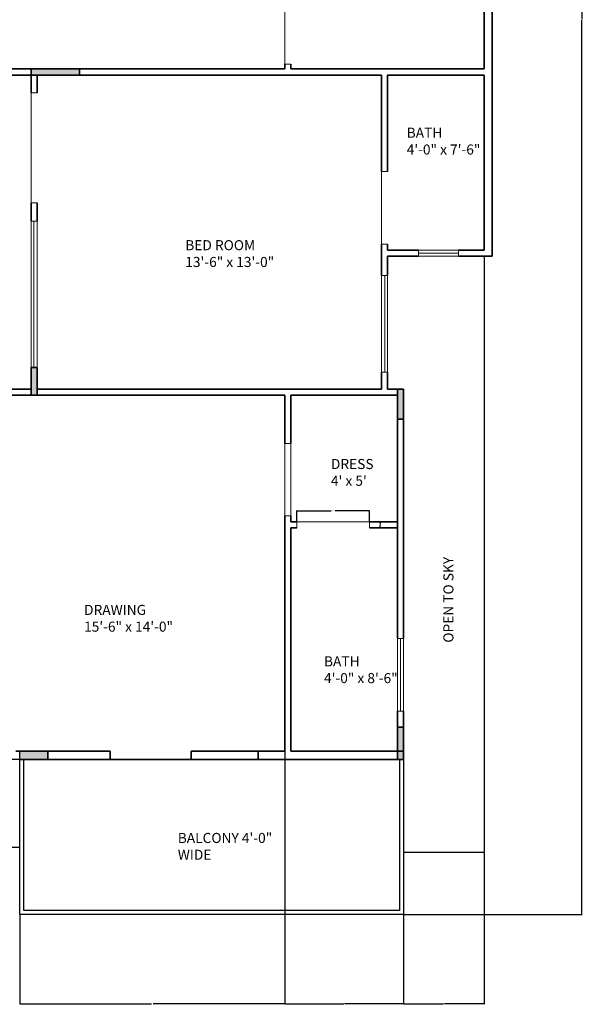
# Model space of a CAD drawing. Units: inches. Extents: x 1002 to 1561, y 1016 to 1994.
# Tile 7 of 8: x 1282 to 1561, y 1016 to 1505. Entities that reach past the tile are written whole.
import ezdxf

# ---------------------------------------------------------------- set-up
doc = ezdxf.new("R2010")
doc.units = ezdxf.units.IN
doc.header["$MEASUREMENT"] = 0
for name, color, linetype, lineweight in [('A-ANNO-DIMS', 2, 'Continuous', 18), ('A-AREA-IDEN', 7, 'Continuous', 18), ('A-WALL', 7, 'Continuous', 35), ('A-WALL-PATT', 7, 'Continuous', 13)]:
    doc.layers.add(name, color=color, linetype=linetype, lineweight=lineweight)
for name, color, linetype, lineweight, true_color in [('A-DOOR', 30, 'Continuous', 18, 0xf8991e), ('A-FLOR-EDGE', 217, 'Continuous', 25, 0x93278f), ('A-GLAZ', 217, 'Continuous', 18, 0x93278f)]:
    doc.layers.add(name, color=color, linetype=linetype, lineweight=lineweight, true_color=true_color)
doc.styles.get("Standard").update_dxf_attribs({"font": 'arial.ttf'})
doc.dimstyles.get("Standard").update_dxf_attribs({"dimtxt": 0.18, "dimasz": 0.18, "dimexe": 0.18, "dimexo": 0.0625, "dimgap": 0.09, "dimtad": 0, "dimtih": 1, "dimtoh": 1, "dimdec": 4, "dimzin": 0, "dimdsep": 46, "dimtxsty": 'Standard', "dimcen": 0.09, "dimadec": 0, "dimazin": 0, "dimtfac": 1, "dimtdec": 4, "dimtofl": 0, "dimtmove": 0, "dimatfit": 3, "dimfxl": 1, "dimtolj": 1, "dimtzin": 0, "dimarcsym": 0})

# ---------------------------------------------------------------- blocks, each defined once
blk = doc.blocks.new('DOOR-OPENING-36IN')
for p, q in [((0, 36), (3, 36)), ((0, 36), (0, 0)), ((0, 0), (3, 0))]:
    blk.add_line(p, q)
blk = doc.blocks.new('*D3')
at = {"layer": 'A-ANNO-DIMS', "color": 0, "lineweight": -2, "transparency": 16777216}
for p, q in [((1419.43, 1255.57), (1419.43, 1261.09)), ((1419.61, 1260.91), (1436.5, 1260.91)), ((1455.25, 1260.91), (1438.37, 1260.91)), ((1455.43, 1255.57), (1455.43, 1261.09))]:
    blk.add_line(p, q, dxfattribs=at)
at = {"layer": 'A-ANNO-DIMS', "color": 0, "transparency": 16777216}
for points in [[(1419.61, 1260.94), (1419.61, 1260.88), (1419.43, 1260.91)], [(1455.25, 1260.94), (1455.25, 1260.88), (1455.43, 1260.91)]]:
    blk.add_solid(points, dxfattribs=at)
at = {"layer": 'Defpoints', "color": 0, "transparency": 16777216}
for p in [(1455.43, 1260.91), (1419.43, 1255.51), (1455.43, 1255.51)]:
    blk.add_point(p, dxfattribs=at)
at = {"layer": 'A-ANNO-DIMS', "color": 0, "transparency": 16777216, "insert": (1437.43, 1260.91), "char_height": 0.18, "attachment_point": 5}
blk.add_mtext('\\A1;DOOR 36 TYP.', dxfattribs=at)
blk = doc.blocks.new('*D4')
at = {"layer": 'A-ANNO-DIMS', "color": 0, "lineweight": -2, "transparency": 16777216}
for p, q in [((1455.5, 1255.51), (1461.01, 1255.51)), ((1455.5, 1252.51), (1461.01, 1252.51)), ((1460.83, 1255.33), (1460.83, 1254.19)), ((1460.83, 1252.69), (1460.83, 1253.83))]:
    blk.add_line(p, q, dxfattribs=at)
at = {"layer": 'A-ANNO-DIMS', "color": 0, "transparency": 16777216}
for points in [[(1460.8, 1255.33), (1460.86, 1255.33), (1460.83, 1255.51)], [(1460.8, 1252.69), (1460.86, 1252.69), (1460.83, 1252.51)]]:
    blk.add_solid(points, dxfattribs=at)
at = {"layer": 'Defpoints', "color": 0, "transparency": 16777216}
for p in [(1455.43, 1255.51), (1455.43, 1252.51), (1460.83, 1252.51)]:
    blk.add_point(p, dxfattribs=at)
at = {"layer": 'A-ANNO-DIMS', "color": 0, "transparency": 16777216, "insert": (1460.83, 1254.01), "char_height": 0.18, "attachment_point": 5}
blk.add_mtext('\\A1;3 TYP.', dxfattribs=at)
blk = doc.blocks.new('*D8')
at = {"layer": 'A-ANNO-DIMS', "color": 0, "lineweight": -2, "transparency": 16777216}
for p, q in [((1516.5, 1949.51), (1561.12, 1949.51)), ((1560.94, 1949.33), (1560.94, 1505.18)), ((1560.94, 1060.67), (1560.94, 1504.82)), ((1472.5, 1060.49), (1561.12, 1060.49))]:
    blk.add_line(p, q, dxfattribs=at)
at = {"layer": 'A-ANNO-DIMS', "color": 0, "transparency": 16777216}
for points in [[(1560.91, 1949.33), (1560.97, 1949.33), (1560.94, 1949.51)], [(1560.91, 1060.67), (1560.97, 1060.67), (1560.94, 1060.49)]]:
    blk.add_solid(points, dxfattribs=at)
at = {"layer": 'Defpoints', "color": 0, "transparency": 16777216}
for p in [(1516.43, 1949.51), (1560.94, 1949.51), (1472.43, 1060.49)]:
    blk.add_point(p, dxfattribs=at)
at = {"layer": 'A-ANNO-DIMS', "color": 0, "transparency": 16777216, "insert": (1560.94, 1505), "char_height": 0.18, "attachment_point": 5}
blk.add_mtext('\\A1;889', dxfattribs=at)
blk = doc.blocks.new('*D19')
at = {"layer": 'A-ANNO-DIMS', "color": 0, "lineweight": -2, "transparency": 16777216}
for p, q in [((1413.43, 1141.45), (1413.43, 1015.8)), ((1281.79, 1060.43), (1281.79, 1015.8)), ((1281.97, 1015.98), (1347.16, 1015.98)), ((1413.25, 1015.98), (1348.07, 1015.98))]:
    blk.add_line(p, q, dxfattribs=at)
at = {"layer": 'A-ANNO-DIMS', "color": 0, "transparency": 16777216}
for points in [[(1281.97, 1016.01), (1281.97, 1015.95), (1281.79, 1015.98)], [(1413.25, 1016.01), (1413.25, 1015.95), (1413.43, 1015.98)]]:
    blk.add_solid(points, dxfattribs=at)
at = {"layer": 'Defpoints', "color": 0, "transparency": 16777216}
for p in [(1413.43, 1141.51), (1281.79, 1060.49), (1413.43, 1015.98)]:
    blk.add_point(p, dxfattribs=at)
at = {"layer": 'A-ANNO-DIMS', "color": 0, "transparency": 16777216, "insert": (1347.61, 1015.98), "char_height": 0.18, "attachment_point": 5}
blk.add_mtext('\\A1;131.64', dxfattribs=at)
blk = doc.blocks.new('*D20')
at = {"layer": 'A-ANNO-DIMS', "color": 0, "lineweight": -2, "transparency": 16777216}
for p, q in [((1413.43, 1141.45), (1413.43, 1015.8)), ((1472.43, 1060.43), (1472.43, 1015.8)), ((1413.61, 1015.98), (1442.71, 1015.98)), ((1472.25, 1015.98), (1443.15, 1015.98))]:
    blk.add_line(p, q, dxfattribs=at)
at = {"layer": 'A-ANNO-DIMS', "color": 0, "transparency": 16777216}
for points in [[(1413.61, 1016.01), (1413.61, 1015.95), (1413.43, 1015.98)], [(1472.25, 1016.01), (1472.25, 1015.95), (1472.43, 1015.98)]]:
    blk.add_solid(points, dxfattribs=at)
at = {"layer": 'Defpoints', "color": 0, "transparency": 16777216}
for p in [(1413.43, 1141.51), (1472.43, 1060.49), (1472.43, 1015.98)]:
    blk.add_point(p, dxfattribs=at)
at = {"layer": 'A-ANNO-DIMS', "color": 0, "transparency": 16777216, "insert": (1442.93, 1015.98), "char_height": 0.18, "attachment_point": 5}
blk.add_mtext('\\A1;59', dxfattribs=at)
blk = doc.blocks.new('*D21')
at = {"layer": 'A-ANNO-DIMS', "color": 0, "lineweight": -2, "transparency": 16777216}
for p, q in [((1512.43, 1091.11), (1512.43, 1015.8)), ((1472.43, 1060.43), (1472.43, 1015.8)), ((1472.61, 1015.98), (1492.21, 1015.98)), ((1512.25, 1015.98), (1492.66, 1015.98))]:
    blk.add_line(p, q, dxfattribs=at)
at = {"layer": 'A-ANNO-DIMS', "color": 0, "transparency": 16777216}
for points in [[(1472.61, 1016.01), (1472.61, 1015.95), (1472.43, 1015.98)], [(1512.25, 1016.01), (1512.25, 1015.95), (1512.43, 1015.98)]]:
    blk.add_solid(points, dxfattribs=at)
at = {"layer": 'Defpoints', "color": 0, "transparency": 16777216}
for p in [(1512.43, 1091.18), (1472.43, 1060.49), (1512.43, 1015.98)]:
    blk.add_point(p, dxfattribs=at)
at = {"layer": 'A-ANNO-DIMS', "color": 0, "transparency": 16777216, "insert": (1492.43, 1015.98), "char_height": 0.18, "attachment_point": 5}
blk.add_mtext('\\A1;40', dxfattribs=at)

msp = doc.modelspace()

# ---------------------------------------------------------------- hatches: boundary and pattern name
at = {"layer": 'A-WALL-PATT'}
h = msp.add_hatch(color=256, dxfattribs=at)
h.dxf.hatch_style = 1
h.paths.add_polyline_path([(1206.434, 1924.784), (1203.434, 1924.784), (1203.434, 1898.155), (1206.434, 1898.155)])
h.paths.add_polyline_path([(1326.434, 1925.745), (1323.434, 1925.745), (1323.434, 1900.458), (1326.434, 1900.458)])
h.paths.add_polyline_path([(1290.434, 1840.51), (1287.434, 1840.51), (1287.434, 1837.51), (1287.434, 1823.284), (1290.434, 1823.284)])
h.paths.add_polyline_path([(1287.434, 1840.51), (1285.684, 1840.51), (1285.684, 1837.51), (1287.434, 1837.51)])
h.paths.add_polyline_path([(1233.434, 1840.51), (1230.434, 1840.51), (1230.434, 1823.284), (1233.434, 1823.284)])
h.paths.add_polyline_path([(1235.119, 1840.51), (1233.434, 1840.51), (1233.434, 1837.51), (1235.119, 1837.51)])
h.paths.add_polyline_path([(1050.434, 1837.51), (1050.434, 1840.51), (1046.434, 1840.51), (1046.434, 1814.619), (1050.434, 1814.619)])
h.paths.add_polyline_path([(1050.434, 1682.088), (1046.434, 1682.088), (1046.434, 1648.51), (1046.434, 1645.51), (1050.434, 1645.51), (1050.434, 1648.51)])
h.paths.add_polyline_path([(1233.434, 1648.51), (1211.636, 1648.51), (1211.636, 1645.51), (1233.434, 1645.51)])
h.paths.add_polyline_path([(1307.549, 1648.51), (1287.434, 1648.51), (1287.434, 1645.51), (1307.549, 1645.51)])
h.paths.add_polyline_path([(1516.434, 1927.595), (1512.434, 1927.595), (1512.434, 1896.846), (1516.434, 1896.846)])
h.paths.add_polyline_path([(1516.434, 1840.51), (1512.434, 1840.51), (1512.434, 1816.31), (1516.434, 1816.31)])
h.paths.add_polyline_path([(1516.434, 1686.827), (1512.434, 1686.827), (1512.434, 1645.51), (1516.434, 1645.51)])
h.paths.add_polyline_path([(1472.434, 1321.51), (1469.434, 1321.51), (1469.434, 1306.51), (1472.434, 1306.51)])
h.paths.add_polyline_path([(1295.733, 1141.51), (1281.793, 1141.51), (1281.793, 1137.51), (1295.733, 1137.51)])
h.paths.add_polyline_path([(1239.434, 1321.51), (1230.434, 1321.51), (1230.434, 1318.51), (1239.434, 1318.51)])
h.paths.add_polyline_path([(1290.434, 1332.122), (1287.434, 1332.122), (1287.434, 1318.51), (1290.434, 1318.51)])
h.paths.add_polyline_path([(1311.434, 1480.51), (1287.434, 1480.51), (1287.434, 1477.51), (1311.434, 1477.51)])
h.paths.add_polyline_path([(1050.434, 1480.51), (1046.434, 1480.51), (1046.434, 1468.51), (1050.434, 1468.51)])
h.paths.add_polyline_path([(1050.434, 1321.51), (1046.434, 1321.51), (1046.434, 1309.51), (1050.434, 1309.51)])
h.paths.add_polyline_path([(1233.434, 1192.382), (1230.434, 1192.382), (1230.434, 1168.702), (1233.434, 1168.702)])
h.paths.add_polyline_path([(1050.434, 1137.51), (1046.434, 1137.51), (1046.434, 1119.51), (1050.434, 1119.51)])
h.paths.add_polyline_path([(1472.434, 1153.51), (1469.434, 1153.51), (1469.434, 1141.51), (1472.434, 1141.51)])
h.paths.add_polyline_path([(1472.434, 1141.51), (1469.434, 1141.51), (1469.434, 1137.51), (1472.434, 1137.51)])

# ---------------------------------------------------------------- linework, layer by layer
at = {"layer": 'A-DOOR'}
for p, q in [((1413.434, 1482.91), (1413.434, 1516.898)), ((1413.434, 1482.91), (1416.434, 1482.91)), ((1287.434, 1468.601), (1290.434, 1468.601)), ((1287.434, 1468.601), (1287.434, 1413.931)), ((1290.434, 1413.931), (1287.434, 1413.931)), ((1413.434, 1294.51), (1416.434, 1294.51)), ((1413.434, 1294.51), (1413.434, 1258.51)), ((1416.434, 1294.51), (1413.434, 1294.51)), ((1416.434, 1258.51), (1416.434, 1294.51)), ((1413.434, 1258.51), (1416.434, 1258.51)), ((1413.434, 1258.51), (1416.434, 1258.51))]:
    msp.add_line(p, q, dxfattribs=at)
at = {"layer": 'A-FLOR-EDGE'}
for p, q in [((1512.434, 1387.51), (1512.434, 1091.177)), ((1281.793, 1060.49), (1281.793, 1141.51)), ((1281.793, 1137.51), (1233.649, 1137.51)), ((1283.793, 1062.49), (1283.793, 1137.51)), ((1470.434, 1137.51), (1470.434, 1062.49)), ((1472.434, 1137.51), (1472.434, 1060.49)), ((1281.793, 1093.652), (1046.434, 1093.652)), ((1512.434, 1091.177), (1472.434, 1091.177)), ((1470.434, 1062.49), (1283.793, 1062.49)), ((1472.434, 1060.49), (1281.793, 1060.49))]:
    msp.add_line(p, q, dxfattribs=at)
at = {"layer": 'A-GLAZ'}
for p, q in [((1287.434, 1404.884), (1290.434, 1404.884)), ((1287.434, 1404.884), (1287.434, 1332.122)), ((1290.434, 1404.884), (1288.885, 1404.884)), ((1288.885, 1404.884), (1288.885, 1332.122)), ((1290.434, 1332.122), (1290.434, 1404.884)), ((1479.744, 1390.51), (1479.744, 1387.51)), ((1499.714, 1390.51), (1479.744, 1390.51)), ((1479.744, 1390.51), (1479.744, 1389.045)), ((1499.714, 1390.51), (1499.714, 1387.51)), ((1499.714, 1387.51), (1499.714, 1390.51)), ((1479.744, 1389.045), (1499.714, 1389.045)), ((1479.744, 1387.51), (1499.714, 1387.51)), ((1461.434, 1377.9), (1464.434, 1377.9)), ((1461.434, 1377.9), (1461.434, 1329.925)), ((1464.434, 1377.9), (1463.078, 1377.9)), ((1463.078, 1377.9), (1463.078, 1329.925)), ((1464.434, 1329.925), (1464.434, 1377.9)), ((1290.434, 1332.122), (1287.434, 1332.122)), ((1461.434, 1329.925), (1464.434, 1329.925)), ((1461.434, 1329.925), (1464.434, 1329.925)), ((1472.434, 1197.51), (1469.434, 1197.51)), ((1469.434, 1197.51), (1469.434, 1161.51)), ((1469.434, 1197.51), (1470.916, 1197.51)), ((1472.434, 1197.51), (1470.916, 1197.51)), ((1470.916, 1197.51), (1470.916, 1161.51)), ((1472.434, 1161.51), (1472.434, 1197.51)), ((1472.434, 1161.51), (1469.434, 1161.51)), ((1469.434, 1161.51), (1472.434, 1161.51))]:
    msp.add_line(p, q, dxfattribs=at)
at = {"layer": 'A-WALL'}
for p, q in [((1512.434, 1945.51), (1512.434, 1480.51)), ((1516.434, 1645.51), (1516.434, 1387.504)), ((1413.434, 1480.51), (1413.434, 1482.91)), ((1416.434, 1480.51), (1416.434, 1482.91)), ((1234.302, 1480.51), (1287.434, 1480.51)), ((1234.302, 1477.51), (1287.434, 1477.51)), ((1287.434, 1477.51), (1287.434, 1480.51)), ((1287.434, 1468.601), (1287.434, 1480.51)), ((1287.434, 1480.51), (1413.434, 1480.51)), ((1287.434, 1477.51), (1461.434, 1477.51)), ((1290.434, 1468.601), (1290.434, 1477.51)), ((1311.434, 1477.51), (1311.434, 1480.51)), ((1416.434, 1480.51), (1512.434, 1480.51)), ((1461.434, 1477.51), (1461.434, 1429.51)), ((1464.434, 1477.51), (1464.434, 1429.51)), ((1464.434, 1477.51), (1512.434, 1477.51)), ((1512.434, 1477.51), (1512.434, 1390.51)), ((1287.434, 1404.884), (1287.434, 1413.931)), ((1290.434, 1404.884), (1290.434, 1413.931)), ((1461.434, 1393.51), (1461.434, 1377.9)), ((1461.434, 1390.51), (1461.434, 1387.51)), ((1464.434, 1393.51), (1464.434, 1390.51)), ((1464.434, 1390.51), (1479.744, 1390.51)), ((1499.714, 1390.51), (1512.434, 1390.51)), ((1464.434, 1387.51), (1479.744, 1387.51)), ((1464.434, 1387.51), (1464.434, 1377.9)), ((1499.714, 1387.51), (1512.434, 1387.51)), ((1516.434, 1387.504), (1512.434, 1387.504)), ((1287.434, 1318.51), (1287.434, 1332.122)), ((1287.434, 1332.122), (1290.434, 1332.122)), ((1290.434, 1318.51), (1290.434, 1332.122)), ((1461.434, 1329.925), (1461.434, 1321.51)), ((1464.434, 1329.925), (1464.434, 1321.51)), ((1275.434, 1321.51), (1287.434, 1321.51)), ((1287.434, 1318.51), (1287.434, 1321.51)), ((1290.434, 1321.51), (1461.434, 1321.51)), ((1464.434, 1321.51), (1472.434, 1321.51)), ((1469.434, 1321.51), (1469.434, 1197.51)), ((1472.434, 1321.51), (1472.434, 1197.51)), ((1275.434, 1318.51), (1413.434, 1318.51)), ((1413.434, 1294.51), (1413.434, 1318.51)), ((1416.434, 1318.51), (1469.434, 1318.51)), ((1416.434, 1294.51), (1416.434, 1318.51)), ((1469.434, 1306.51), (1472.434, 1306.51)), ((1413.434, 1141.51), (1413.434, 1258.51)), ((1416.434, 1255.51), (1416.434, 1258.51)), ((1416.434, 1255.51), (1419.434, 1255.51)), ((1416.434, 1141.51), (1416.434, 1252.51)), ((1416.434, 1252.51), (1419.434, 1252.51)), ((1455.434, 1255.51), (1469.434, 1255.51)), ((1455.434, 1252.51), (1469.434, 1252.51)), ((1469.434, 1161.51), (1469.434, 1137.51)), ((1472.434, 1161.51), (1472.434, 1137.51)), ((1472.434, 1153.51), (1469.434, 1153.51)), ((1279.793, 1141.51), (1281.793, 1141.51)), ((1281.793, 1141.51), (1326.715, 1141.51)), ((1295.733, 1141.51), (1295.733, 1137.51)), ((1326.715, 1137.51), (1326.715, 1141.51)), ((1366.852, 1141.51), (1366.852, 1137.51)), ((1366.852, 1141.51), (1400.182, 1141.51)), ((1400.182, 1137.51), (1400.182, 1141.51)), ((1413.434, 1141.51), (1400.182, 1141.51)), ((1472.434, 1141.51), (1416.434, 1141.51)), ((1281.793, 1137.51), (1400.182, 1137.51)), ((1472.434, 1137.51), (1400.182, 1137.51))]:
    msp.add_line(p, q, dxfattribs=at)

# ---------------------------------------------------------------- block references
at = {"layer": 'A-DOOR'}
msp.add_blockref('DOOR-OPENING-36IN', (1461.434, 1393.51), dxfattribs=at)
at = {"layer": 'A-DOOR', "rotation": 269.9999999999999}
msp.add_blockref('DOOR-OPENING-36IN', (1419.433, 1255.51), dxfattribs=at)

# ---------------------------------------------------------------- texts
at = {"layer": 'A-AREA-IDEN', "char_height": 5, "attachment_point": 1}
for s, insert in [('BATH\\P4\'-0" x 7\'-6"', (1473.955, 1451.344)), ('BED ROOM\\P13\'-6" x 13\'-0"', (1364.008, 1395.466)), ("DRESS\\P4' x 5'", (1436.329, 1286.745)), ('DRAWING\\P15\'-6" x 14\'-0"', (1313.773, 1214.264)), ('BATH\\P4\'-0" x 8\'-6"', (1432.893, 1188.705)), ('BALCONY 4\'-0" WIDE', (1360.287, 1100.946))]:
    msp.add_mtext_dynamic_manual_height_columns(s, width=50.5101, gutter_width=1, heights=[0], dxfattribs=dict(at, insert=insert))
at = {"layer": 'A-AREA-IDEN', "insert": (1492.169, 1195.474), "char_height": 5, "attachment_point": 1, "rotation": 90}
msp.add_mtext_dynamic_manual_height_columns('OPEN TO SKY', width=50.5101, gutter_width=1, heights=[0], dxfattribs=at)

# ---------------------------------------------------------------- dimensions: what is measured, and where the dimension line sits
at = {"layer": 'A-ANNO-DIMS'}
dim = msp.add_linear_dim(base=(1560.944, 1949.51), p1=(1472.434, 1060.49), p2=(1516.434, 1949.51), angle=90, dimstyle='Standard', override={"dimdec": 0, "dimlfac": 1, "dimrnd": 0, "dimzin": 0, "dimdsep": 46, "dimlunit": 2}, dxfattribs=at)
dim.commit()
dim.dimension.update_dxf_attribs({"geometry": '*D8', "text_midpoint": (1560.944, 1505)})
dim = msp.add_linear_dim(base=(1455.434, 1260.91), p1=(1419.434, 1255.51), p2=(1455.434, 1255.51), text='DOOR <> TYP.', dimstyle='Standard', override={"dimdec": 0, "dimlfac": 1, "dimrnd": 0, "dimzin": 0, "dimdsep": 46, "dimlunit": 2}, dxfattribs=at)
dim.commit()
dim.dimension.update_dxf_attribs({"geometry": '*D3', "text_midpoint": (1437.434, 1260.91)})
dim = msp.add_linear_dim(base=(1460.834, 1252.51), p1=(1455.434, 1255.51), p2=(1455.434, 1252.51), angle=270, text='<> TYP.', dimstyle='Standard', override={"dimdec": 0, "dimlfac": 1, "dimrnd": 0, "dimzin": 0, "dimdsep": 46, "dimlunit": 2}, dxfattribs=at)
dim.commit()
dim.dimension.update_dxf_attribs({"geometry": '*D4', "text_midpoint": (1460.834, 1254.01)})
for base, p1, p2, override, picture, middle in [((1413.434, 1015.98), (1281.793, 1060.49), (1413.434, 1141.51), {"dimdec": 2, "dimlfac": 1, "dimrnd": 0, "dimzin": 0, "dimdsep": 46, "dimlunit": 2}, '*D19', (1347.613, 1015.98)), ((1472.434, 1015.98), (1413.434, 1141.51), (1472.434, 1060.49), {"dimdec": 0, "dimlfac": 1, "dimrnd": 0, "dimzin": 0, "dimdsep": 46, "dimlunit": 2}, '*D20', (1442.934, 1015.98)), ((1512.434, 1015.98), (1472.434, 1060.49), (1512.434, 1091.177), {"dimdec": 0, "dimlfac": 1, "dimrnd": 0, "dimzin": 0, "dimdsep": 46, "dimlunit": 2}, '*D21', (1492.434, 1015.98))]:
    dim = msp.add_linear_dim(base=base, p1=p1, p2=p2, dimstyle='Standard', override=override, dxfattribs=at)
    dim.commit()
    dim.dimension.update_dxf_attribs({"geometry": picture, "text_midpoint": middle})

doc.saveas('drawing.dxf')
